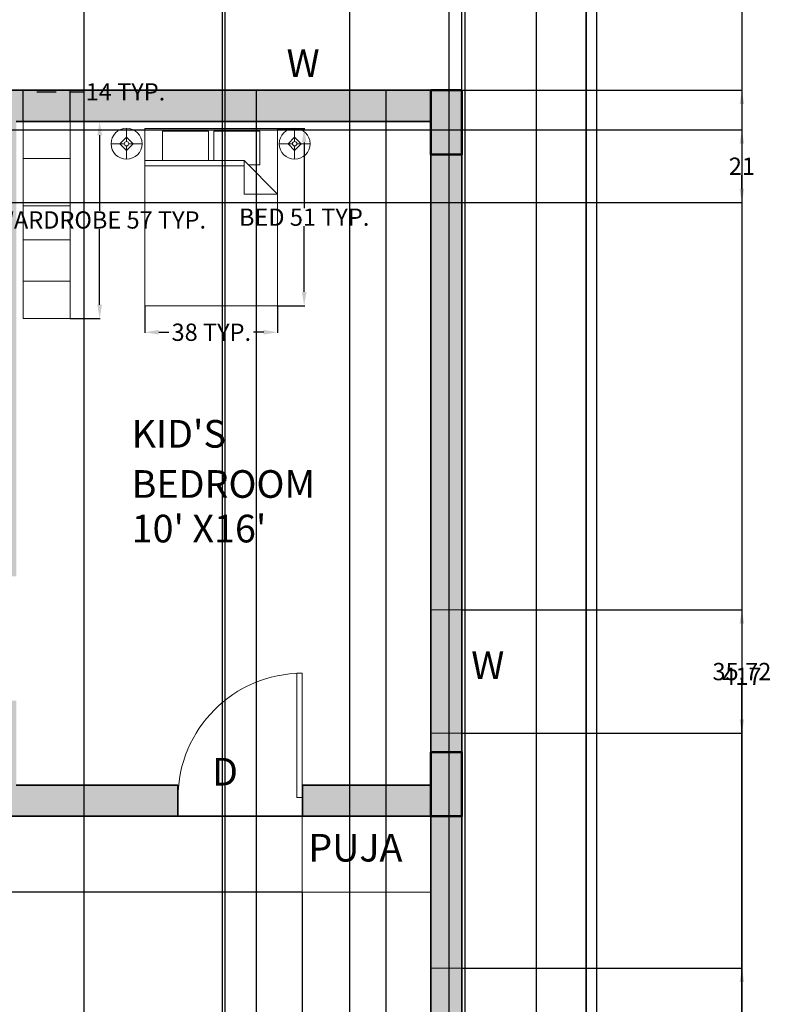
# Model space of a CAD drawing. Units: inches. Extents: x 460 to 1030, y -658 to 271.
# Tile 9 of 10: x 813 to 1030, y -174 to 111. Entities that reach past the tile are written whole.
import ezdxf

# ---------------------------------------------------------------- set-up
doc = ezdxf.new("R2010")
doc.units = ezdxf.units.IN
doc.header["$MEASUREMENT"] = 0
for name, color, linetype, lineweight in [('A-ANNO-DIMS', 2, 'Continuous', 18), ('A-ANNO-TEXT', 7, 'Continuous', 18), ('A-AREA-IDEN', 7, 'Continuous', 25), ('A-COLS', 7, 'Continuous', 50), ('A-DOOR', 3, 'Continuous', 20), ('A-FLOR-CASE', 9, 'Continuous', 18), ('A-FURN', 8, 'Continuous', 18), ('A-GLAZ', 4, 'Continuous', 20), ('A-GLAZ-PATT', 4, 'Continuous', 13), ('A-WALL', 7, 'Continuous', 35), ('A-WALL-PATT', 5, 'Continuous', 13), ('C-PROP', 7, 'Continuous', 25)]:
    doc.layers.add(name, color=color, linetype=linetype, lineweight=lineweight)
doc.layers.add('A-COLS-PATT', color=7, linetype='Continuous', lineweight=13, true_color=0xffffff)
doc.styles.get("Standard").update_dxf_attribs({"font": 'arial.ttf'})
doc.dimstyles.get("Standard").update_dxf_attribs({"dimtxt": 5, "dimasz": 4, "dimexe": 0.18, "dimexo": 0.0625, "dimgap": 0.09, "dimtad": 0, "dimtih": 1, "dimtoh": 1, "dimdec": 1, "dimzin": 0, "dimdsep": 46, "dimlunit": 4, "dimtxsty": 'Standard', "dimcen": 0.09, "dimadec": 0, "dimazin": 0, "dimtfac": 1, "dimtdec": 1, "dimtofl": 0, "dimtmove": 0, "dimatfit": 3, "dimfxl": 1, "dimtolj": 1, "dimtzin": 0, "dimarcsym": 0})

# ---------------------------------------------------------------- blocks, each defined once
blk = doc.blocks.new('Bed - Queen')
for p, q in [((0, -80.00003), (0, 0)), ((0, 0), (59.99999, 0)), ((59.99999, 0), (59.99999, -80.00003)), ((7.99999, -1.2), (28.79998, -1.2)), ((7.99999, -14.4), (7.99999, -1.2)), ((28.79998, -1.2), (28.79998, -14.4)), ((31.19999, -1.2), (51.99999, -1.2)), ((31.19999, -14.4), (31.19999, -1.2)), ((51.99999, -1.2), (51.99999, -16.4)), ((0, -14.4), (44.8, -14.4)), ((44.8, -16.8), (0, -16.8)), ((59.99999, -29.6), (44.8, -14.4)), ((44.8, -14.4), (44.8, -29.6)), ((51.99999, -16.4), (46.79936, -16.4)), ((44.8, -29.6), (59.99999, -29.6)), ((59.99999, -80.00003), (0, -80.00003))]:
    blk.add_line(p, q)
blk = doc.blocks.new('Lamp - Table')
for p, q in [((0, 7), (0, 1)), ((-1, 0), (-7, 0)), ((0, 3), (-3, 0)), ((-3, 0), (0, -3)), ((3, 0), (0, 3)), ((0, -3), (3, 0)), ((1, 0), (7, 0)), ((0, -1), (0, -7))]:
    blk.add_line(p, q)
for radius in [7, 1]:
    blk.add_circle((0, 0), radius)
blk = doc.blocks.new('*U2')
for p, q in [((0, 0), (0, -6)), ((40, 0), (40, -6))]:
    blk.add_line(p, q)
blk.add_lwpolyline([(0, 0), (0, 40), (1.75, 40), (1.75, 0)], close=True)
blk.add_arc((0, 0), 40, 0, 90)
blk = doc.blocks.new('BEDROOM-STORAGE-UNIT')
for p, q in [((10.68, 0), (10.68, -13.59)), ((24.45, 0), (24.45, -13.59)), ((34.21, 0), (34.21, -13.59)), ((46.22, 0), (46.22, -13.59))]:
    blk.add_line(p, q)
blk.add_lwpolyline([(0, 0), (57.01, 0), (57.01, -13.59), (0, -13.59)], close=True)
blk = doc.blocks.new('COL-RECT-TYPE-A')
blk.add_lwpolyline([(0, 0), (9, 0), (9, -18.58), (0, -18.58)], close=True)
blk = doc.blocks.new('*D25')
at = {"layer": 'A-ANNO-DIMS', "color": 0, "lineweight": -2, "transparency": 16777216}
for p, q in [((887.53, 79.18), (895.33, 79.18)), ((895.15, 75.18), (895.15, 56.22)), ((895.15, 31.97), (895.15, 50.93)), ((887.53, 27.97), (895.33, 27.97))]:
    blk.add_line(p, q, dxfattribs=at)
at = {"layer": 'A-ANNO-DIMS', "color": 0, "transparency": 16777216}
for points in [[(894.48, 75.18), (895.82, 75.18), (895.15, 79.18)], [(894.48, 31.97), (895.82, 31.97), (895.15, 27.97)]]:
    blk.add_solid(points, dxfattribs=at)
at = {"layer": 'Defpoints', "color": 0, "transparency": 16777216}
for p in [(887.47, 79.18), (895.15, 79.18), (887.47, 27.97)]:
    blk.add_point(p, dxfattribs=at)
at = {"layer": 'A-ANNO-DIMS', "color": 0, "transparency": 16777216, "insert": (895.15, 53.58), "char_height": 5, "attachment_point": 5}
blk.add_mtext('\\A1;BED 51 TYP.', dxfattribs=at)
blk = doc.blocks.new('*D26')
at = {"layer": 'A-ANNO-DIMS', "color": 0, "lineweight": -2, "transparency": 16777216}
for p, q in [((849.06, 27.91), (849.06, 20.11)), ((887.47, 27.91), (887.47, 20.11)), ((853.06, 20.29), (856.01, 20.29)), ((883.47, 20.29), (880.52, 20.29))]:
    blk.add_line(p, q, dxfattribs=at)
at = {"layer": 'A-ANNO-DIMS', "color": 0, "transparency": 16777216}
for points in [[(853.06, 20.96), (853.06, 19.62), (849.06, 20.29)], [(883.47, 20.96), (883.47, 19.62), (887.47, 20.29)]]:
    blk.add_solid(points, dxfattribs=at)
at = {"layer": 'Defpoints', "color": 0, "transparency": 16777216}
for p in [(849.06, 27.97), (887.47, 27.97), (887.47, 20.29)]:
    blk.add_point(p, dxfattribs=at)
at = {"layer": 'A-ANNO-DIMS', "color": 0, "transparency": 16777216, "insert": (868.27, 20.29), "char_height": 5, "attachment_point": 5}
blk.add_mtext('\\A1;38 TYP.', dxfattribs=at)
blk = doc.blocks.new('*D27')
at = {"layer": 'A-ANNO-DIMS', "color": 0, "lineweight": -2, "transparency": 16777216}
for p, q in [((827.46, 81.27), (836.13, 81.27)), ((835.95, 77.27), (835.95, 55.44)), ((835.95, 28.26), (835.95, 50.09)), ((827.46, 24.26), (836.13, 24.26))]:
    blk.add_line(p, q, dxfattribs=at)
at = {"layer": 'A-ANNO-DIMS', "color": 0, "transparency": 16777216}
for points in [[(835.28, 77.27), (836.62, 77.27), (835.95, 81.27)], [(835.28, 28.26), (836.62, 28.26), (835.95, 24.26)]]:
    blk.add_solid(points, dxfattribs=at)
at = {"layer": 'Defpoints', "color": 0, "transparency": 16777216}
for p in [(827.4, 81.27), (827.4, 24.26), (835.95, 24.26)]:
    blk.add_point(p, dxfattribs=at)
at = {"layer": 'A-ANNO-DIMS', "color": 0, "transparency": 16777216, "insert": (835.95, 52.77), "char_height": 5, "attachment_point": 5}
blk.add_mtext('\\A1;WARDROBE 57 TYP.', dxfattribs=at)
blk = doc.blocks.new('*D28')
at = {"layer": 'A-ANNO-DIMS', "color": 0, "lineweight": -2, "transparency": 16777216}
for p, q in [((813.8, 81.34), (813.8, 90.01)), ((817.8, 89.83), (823.4, 89.83)), ((827.4, 81.34), (827.4, 90.01)), ((827.4, 89.83), (831.4, 89.83))]:
    blk.add_line(p, q, dxfattribs=at)
at = {"layer": 'A-ANNO-DIMS', "color": 0, "transparency": 16777216}
for points in [[(817.8, 90.49), (817.8, 89.16), (813.8, 89.83)], [(823.4, 90.49), (823.4, 89.16), (827.4, 89.83)]]:
    blk.add_solid(points, dxfattribs=at)
at = {"layer": 'Defpoints', "color": 0, "transparency": 16777216}
for p in [(827.4, 89.83), (813.8, 81.27), (827.4, 81.27)]:
    blk.add_point(p, dxfattribs=at)
at = {"layer": 'A-ANNO-DIMS', "color": 0, "transparency": 16777216, "insert": (843.42, 89.83), "char_height": 5, "attachment_point": 5}
blk.add_mtext('\\A1;14 TYP.', dxfattribs=at)
blk = doc.blocks.new('*D41')
at = {"layer": 'A-ANNO-DIMS', "color": 0, "lineweight": -2, "transparency": 16777216}
for p, q in [((979.86, 129.27), (1022.03, 129.27)), ((1021.85, 125.27), (1021.85, -76.63)), ((1021.85, -283.73), (1021.85, -81.83)), ((940.86, -287.73), (1022.03, -287.73))]:
    blk.add_line(p, q, dxfattribs=at)
at = {"layer": 'A-ANNO-DIMS', "color": 0, "transparency": 16777216}
for points in [[(1021.18, 125.27), (1022.51, 125.27), (1021.85, 129.27)], [(1021.18, -283.73), (1022.51, -283.73), (1021.85, -287.73)]]:
    blk.add_solid(points, dxfattribs=at)
at = {"layer": 'Defpoints', "color": 0, "transparency": 16777216}
for p in [(979.8, 129.27), (1021.85, 129.27), (940.8, -287.73)]:
    blk.add_point(p, dxfattribs=at)
at = {"layer": 'A-ANNO-DIMS', "color": 0, "transparency": 16777216, "insert": (1021.85, -79.23), "char_height": 5, "attachment_point": 5}
blk.add_mtext('\\A1;417', dxfattribs=at)
blk = doc.blocks.new('*D43')
at = {"layer": 'A-ANNO-DIMS', "color": 0, "lineweight": -2, "transparency": 16777216}
for p, q in [((562.8, 90.34), (562.8, 267.89)), ((940.8, 90.34), (940.8, 267.89)), ((566.8, 267.71), (746.18, 267.71)), ((936.8, 267.71), (757.41, 267.71))]:
    blk.add_line(p, q, dxfattribs=at)
at = {"layer": 'A-ANNO-DIMS', "color": 0, "transparency": 16777216}
for points in [[(566.8, 268.38), (566.8, 267.04), (562.8, 267.71)], [(936.8, 268.38), (936.8, 267.04), (940.8, 267.71)]]:
    blk.add_solid(points, dxfattribs=at)
at = {"layer": 'Defpoints', "color": 0, "transparency": 16777216}
for p in [(940.8, 267.71), (562.8, 90.27), (940.8, 90.27)]:
    blk.add_point(p, dxfattribs=at)
at = {"layer": 'A-ANNO-DIMS', "color": 0, "transparency": 16777216, "insert": (751.8, 267.71), "char_height": 5, "attachment_point": 5}
blk.add_mtext('\\A1;378', dxfattribs=at)
blk = doc.blocks.new('*D44')
at = {"layer": 'A-ANNO-DIMS', "color": 0, "lineweight": -2, "transparency": 16777216}
for p, q in [((940.86, 90.27), (1022.03, 90.27)), ((1021.85, 86.27), (1021.85, -195.08)), ((1021.85, -481.73), (1021.85, -200.37)), ((979.86, -485.73), (1022.03, -485.73))]:
    blk.add_line(p, q, dxfattribs=at)
at = {"layer": 'A-ANNO-DIMS', "color": 0, "transparency": 16777216}
for points in [[(1021.18, 86.27), (1022.51, 86.27), (1021.85, 90.27)], [(1021.18, -481.73), (1022.51, -481.73), (1021.85, -485.73)]]:
    blk.add_solid(points, dxfattribs=at)
at = {"layer": 'Defpoints', "color": 0, "transparency": 16777216}
for p in [(940.8, 90.27), (979.8, -485.73), (1021.85, -485.73)]:
    blk.add_point(p, dxfattribs=at)
at = {"layer": 'A-ANNO-DIMS', "color": 0, "transparency": 16777216, "insert": (1021.85, -197.73), "char_height": 5, "attachment_point": 5}
blk.add_mtext('\\A1;576', dxfattribs=at)
blk = doc.blocks.new('*D45')
at = {"layer": 'A-ANNO-DIMS', "color": 0, "lineweight": -2, "transparency": 16777216}
for p, q in [((976.8, 126.21), (976.8, -654.61)), ((940.8, 90.21), (940.8, -654.61)), ((944.8, -654.43), (955.13, -654.43)), ((972.8, -654.43), (962.46, -654.43))]:
    blk.add_line(p, q, dxfattribs=at)
at = {"layer": 'A-ANNO-DIMS', "color": 0, "transparency": 16777216}
for points in [[(944.8, -653.77), (944.8, -655.1), (940.8, -654.43)], [(972.8, -653.77), (972.8, -655.1), (976.8, -654.43)]]:
    blk.add_solid(points, dxfattribs=at)
at = {"layer": 'Defpoints', "color": 0, "transparency": 16777216}
for p in [(976.8, 126.27), (940.8, 90.27), (976.8, -654.43)]:
    blk.add_point(p, dxfattribs=at)
at = {"layer": 'A-ANNO-DIMS', "color": 0, "transparency": 16777216, "insert": (958.8, -654.43), "char_height": 5, "attachment_point": 5}
blk.add_mtext('\\A1;36', dxfattribs=at)
blk = doc.blocks.new('*D46')
at = {"layer": 'A-ANNO-DIMS', "color": 0, "lineweight": -2, "transparency": 16777216}
for p, q in [((936.98, 127.21), (936.98, -654.61)), ((962.32, 127.21), (962.32, -654.61)), ((932.98, -654.43), (928.98, -654.43)), ((966.32, -654.43), (970.32, -654.43))]:
    blk.add_line(p, q, dxfattribs=at)
at = {"layer": 'A-ANNO-DIMS', "color": 0, "transparency": 16777216}
for points in [[(932.98, -653.77), (932.98, -655.1), (936.98, -654.43)], [(966.32, -653.77), (966.32, -655.1), (962.32, -654.43)]]:
    blk.add_solid(points, dxfattribs=at)
at = {"layer": 'Defpoints', "color": 0, "transparency": 16777216}
for p in [(936.98, 127.27), (962.32, 127.27), (962.32, -654.43)]:
    blk.add_point(p, dxfattribs=at)
at = {"layer": 'A-ANNO-DIMS', "color": 0, "transparency": 16777216, "insert": (949.65, -654.43), "char_height": 5, "attachment_point": 5}
blk.add_mtext('\\A1;25.346', dxfattribs=at)
blk = doc.blocks.new('*D47')
at = {"layer": 'A-ANNO-DIMS', "color": 0, "lineweight": -2, "transparency": 16777216}
for p, q in [((962.32, 129.21), (962.32, -654.61)), ((979.8, 129.21), (979.8, -654.61)), ((966.32, -654.43), (975.8, -654.43)), ((979.8, -654.43), (983.8, -654.43))]:
    blk.add_line(p, q, dxfattribs=at)
at = {"layer": 'A-ANNO-DIMS', "color": 0, "transparency": 16777216}
for points in [[(966.32, -653.77), (966.32, -655.1), (962.32, -654.43)], [(975.8, -653.77), (975.8, -655.1), (979.8, -654.43)]]:
    blk.add_solid(points, dxfattribs=at)
at = {"layer": 'Defpoints', "color": 0, "transparency": 16777216}
for p in [(962.32, 129.27), (979.8, 129.27), (979.8, -654.43)]:
    blk.add_point(p, dxfattribs=at)
at = {"layer": 'A-ANNO-DIMS', "color": 0, "transparency": 16777216, "insert": (994.02, -654.43), "char_height": 5, "attachment_point": 5}
blk.add_mtext('\\A1;17.474', dxfattribs=at)
blk = doc.blocks.new('*D48')
at = {"layer": 'A-ANNO-DIMS', "color": 0, "lineweight": -2, "transparency": 16777216}
for p, q in [((799.88, -611.66), (799.88, 267.89)), ((941.7, -611.66), (941.7, 267.89)), ((803.88, 267.71), (860.58, 267.71)), ((937.7, 267.71), (881, 267.71))]:
    blk.add_line(p, q, dxfattribs=at)
at = {"layer": 'A-ANNO-DIMS', "color": 0, "transparency": 16777216}
for points in [[(803.88, 268.38), (803.88, 267.04), (799.88, 267.71)], [(937.7, 268.38), (937.7, 267.04), (941.7, 267.71)]]:
    blk.add_solid(points, dxfattribs=at)
at = {"layer": 'Defpoints', "color": 0, "transparency": 16777216}
for p in [(941.7, 267.71), (799.88, -611.73), (941.7, -611.73)]:
    blk.add_point(p, dxfattribs=at)
at = {"layer": 'A-ANNO-DIMS', "color": 0, "transparency": 16777216, "insert": (870.79, 267.71), "char_height": 5, "attachment_point": 5}
blk.add_mtext('\\A1;141.82', dxfattribs=at)
blk = doc.blocks.new('*D49')
at = {"layer": 'A-ANNO-DIMS', "color": 0, "lineweight": -2, "transparency": 16777216}
for p, q in [((941.7, -608.66), (941.7, 267.89)), ((976.8, -608.66), (976.8, 267.89)), ((945.7, 267.71), (953.15, 267.71)), ((972.8, 267.71), (965.35, 267.71))]:
    blk.add_line(p, q, dxfattribs=at)
at = {"layer": 'A-ANNO-DIMS', "color": 0, "transparency": 16777216}
for points in [[(945.7, 268.38), (945.7, 267.04), (941.7, 267.71)], [(972.8, 268.38), (972.8, 267.04), (976.8, 267.71)]]:
    blk.add_solid(points, dxfattribs=at)
at = {"layer": 'Defpoints', "color": 0, "transparency": 16777216}
for p in [(976.8, 267.71), (941.7, -608.73), (976.8, -608.73)]:
    blk.add_point(p, dxfattribs=at)
at = {"layer": 'A-ANNO-DIMS', "color": 0, "transparency": 16777216, "insert": (959.25, 267.71), "char_height": 5, "attachment_point": 5}
blk.add_mtext('\\A1;35.1', dxfattribs=at)
blk = doc.blocks.new('*D52')
at = {"layer": 'A-ANNO-DIMS', "color": 0, "lineweight": -2, "transparency": 16777216}
for p, q in [((872.3, -281.66), (872.3, 267.89)), ((908.35, -281.66), (908.35, 267.89)), ((876.3, 267.71), (879.84, 267.71)), ((904.35, 267.71), (900.81, 267.71))]:
    blk.add_line(p, q, dxfattribs=at)
at = {"layer": 'A-ANNO-DIMS', "color": 0, "transparency": 16777216}
for points in [[(876.3, 268.38), (876.3, 267.04), (872.3, 267.71)], [(904.35, 268.38), (904.35, 267.04), (908.35, 267.71)]]:
    blk.add_solid(points, dxfattribs=at)
at = {"layer": 'Defpoints', "color": 0, "transparency": 16777216}
for p in [(908.35, 267.71), (872.3, -281.73), (908.35, -281.73)]:
    blk.add_point(p, dxfattribs=at)
at = {"layer": 'A-ANNO-DIMS', "color": 0, "transparency": 16777216, "insert": (890.32, 267.71), "char_height": 5, "attachment_point": 5}
blk.add_mtext('\\A1;36.045', dxfattribs=at)
blk = doc.blocks.new('*D54')
at = {"layer": 'A-ANNO-DIMS', "color": 0, "lineweight": -2, "transparency": 16777216}
for p, q in [((894.61, -141.78), (894.61, -654.61)), ((931.8, -141.78), (931.8, -654.61)), ((898.61, -654.43), (904.68, -654.43)), ((927.8, -654.43), (921.73, -654.43))]:
    blk.add_line(p, q, dxfattribs=at)
at = {"layer": 'A-ANNO-DIMS', "color": 0, "transparency": 16777216}
for points in [[(898.61, -653.77), (898.61, -655.1), (894.61, -654.43)], [(927.8, -653.77), (927.8, -655.1), (931.8, -654.43)]]:
    blk.add_solid(points, dxfattribs=at)
at = {"layer": 'Defpoints', "color": 0, "transparency": 16777216}
for p in [(894.61, -141.72), (931.8, -141.72), (931.8, -654.43)]:
    blk.add_point(p, dxfattribs=at)
at = {"layer": 'A-ANNO-DIMS', "color": 0, "transparency": 16777216, "insert": (913.2, -654.43), "char_height": 5, "attachment_point": 5}
blk.add_mtext('\\A1;37.18', dxfattribs=at)
blk = doc.blocks.new('*D55')
at = {"layer": 'A-ANNO-DIMS', "color": 0, "lineweight": -2, "transparency": 16777216}
for p, q in [((894.56, -119.73), (470.68, -119.73)), ((470.86, -123.73), (470.86, -128.08)), ((470.86, -137.72), (470.86, -133.37)), ((894.55, -141.72), (470.68, -141.72))]:
    blk.add_line(p, q, dxfattribs=at)
at = {"layer": 'A-ANNO-DIMS', "color": 0, "transparency": 16777216}
for points in [[(470.19, -123.73), (471.52, -123.73), (470.86, -119.73)], [(470.19, -137.72), (471.52, -137.72), (470.86, -141.72)]]:
    blk.add_solid(points, dxfattribs=at)
at = {"layer": 'Defpoints', "color": 0, "transparency": 16777216}
for p in [(470.86, -119.73), (894.62, -119.73), (894.61, -141.72)]:
    blk.add_point(p, dxfattribs=at)
at = {"layer": 'A-ANNO-DIMS', "color": 0, "transparency": 16777216, "insert": (470.86, -130.72), "char_height": 5, "attachment_point": 5}
blk.add_mtext('\\A1;21.995', dxfattribs=at)
blk = doc.blocks.new('*D59')
at = {"layer": 'A-ANNO-DIMS', "color": 0, "lineweight": -2, "transparency": 16777216}
for p, q in [((940.86, -60), (1022.03, -60)), ((1021.85, -64), (1021.85, -75.22)), ((1021.85, -91.73), (1021.85, -80.51)), ((940.86, -95.73), (1022.03, -95.73))]:
    blk.add_line(p, q, dxfattribs=at)
at = {"layer": 'A-ANNO-DIMS', "color": 0, "transparency": 16777216}
for points in [[(1021.18, -64), (1022.51, -64), (1021.85, -60)], [(1021.18, -91.73), (1022.51, -91.73), (1021.85, -95.73)]]:
    blk.add_solid(points, dxfattribs=at)
at = {"layer": 'Defpoints', "color": 0, "transparency": 16777216}
for p in [(940.8, -60), (940.8, -95.73), (1021.85, -95.73)]:
    blk.add_point(p, dxfattribs=at)
at = {"layer": 'A-ANNO-DIMS', "color": 0, "transparency": 16777216, "insert": (1021.85, -77.87), "char_height": 5, "attachment_point": 5}
blk.add_mtext('\\A1;35.72', dxfattribs=at)
blk = doc.blocks.new('*D60')
at = {"layer": 'A-ANNO-DIMS', "color": 0, "lineweight": -2, "transparency": 16777216}
for p, q in [((940.86, -163.66), (1022.03, -163.66)), ((1021.85, -167.66), (1021.85, -194.33)), ((1021.85, -226.29), (1021.85, -199.62)), ((940.86, -230.29), (1022.03, -230.29))]:
    blk.add_line(p, q, dxfattribs=at)
at = {"layer": 'A-ANNO-DIMS', "color": 0, "transparency": 16777216}
for points in [[(1021.18, -167.66), (1022.51, -167.66), (1021.85, -163.66)], [(1021.18, -226.29), (1022.51, -226.29), (1021.85, -230.29)]]:
    blk.add_solid(points, dxfattribs=at)
at = {"layer": 'Defpoints', "color": 0, "transparency": 16777216}
for p in [(940.8, -163.66), (940.8, -230.29), (1021.85, -230.29)]:
    blk.add_point(p, dxfattribs=at)
at = {"layer": 'A-ANNO-DIMS', "color": 0, "transparency": 16777216, "insert": (1021.85, -196.98), "char_height": 5, "attachment_point": 5}
blk.add_mtext('\\A1;66.64', dxfattribs=at)
blk = doc.blocks.new('*D69')
at = {"layer": 'A-ANNO-DIMS', "color": 0, "lineweight": -2, "transparency": 16777216}
for p, q in [((881.27, 90.21), (881.27, -654.61)), ((918.77, 90.21), (918.77, -654.61)), ((885.27, -654.43), (893.42, -654.43)), ((914.77, -654.43), (906.62, -654.43))]:
    blk.add_line(p, q, dxfattribs=at)
at = {"layer": 'A-ANNO-DIMS', "color": 0, "transparency": 16777216}
for points in [[(885.27, -653.77), (885.27, -655.1), (881.27, -654.43)], [(914.77, -653.77), (914.77, -655.1), (918.77, -654.43)]]:
    blk.add_solid(points, dxfattribs=at)
at = {"layer": 'Defpoints', "color": 0, "transparency": 16777216}
for p in [(881.27, 90.27), (918.77, 90.27), (918.77, -654.43)]:
    blk.add_point(p, dxfattribs=at)
at = {"layer": 'A-ANNO-DIMS', "color": 0, "transparency": 16777216, "insert": (900.02, -654.43), "char_height": 5, "attachment_point": 5}
blk.add_mtext('\\A1;37.5', dxfattribs=at)
blk = doc.blocks.new('*D71')
at = {"layer": 'A-ANNO-DIMS', "color": 0, "lineweight": -2, "transparency": 16777216}
for p, q in [((831.43, -281.66), (831.43, 267.89)), ((871.46, -281.66), (871.46, 267.89)), ((835.43, 267.71), (840.88, 267.71)), ((867.46, 267.71), (862.01, 267.71))]:
    blk.add_line(p, q, dxfattribs=at)
at = {"layer": 'A-ANNO-DIMS', "color": 0, "transparency": 16777216}
for points in [[(835.43, 268.38), (835.43, 267.04), (831.43, 267.71)], [(867.46, 268.38), (867.46, 267.04), (871.46, 267.71)]]:
    blk.add_solid(points, dxfattribs=at)
at = {"layer": 'Defpoints', "color": 0, "transparency": 16777216}
for p in [(871.46, 267.71), (831.43, -281.73), (871.46, -281.73)]:
    blk.add_point(p, dxfattribs=at)
at = {"layer": 'A-ANNO-DIMS', "color": 0, "transparency": 16777216, "insert": (851.44, 267.71), "char_height": 5, "attachment_point": 5}
blk.add_mtext('\\A1;40.026', dxfattribs=at)
blk = doc.blocks.new('*D73')
at = {"layer": 'A-ANNO-DIMS', "color": 0, "lineweight": -2, "transparency": 16777216}
for p, q in [((748.86, 78.81), (1022.03, 78.81)), ((1021.85, 74.81), (1021.85, 70.92)), ((1021.85, 61.81), (1021.85, 65.71)), ((748.86, 57.81), (1022.03, 57.81))]:
    blk.add_line(p, q, dxfattribs=at)
at = {"layer": 'A-ANNO-DIMS', "color": 0, "transparency": 16777216}
for points in [[(1021.18, 74.81), (1022.51, 74.81), (1021.85, 78.81)], [(1021.18, 61.81), (1022.51, 61.81), (1021.85, 57.81)]]:
    blk.add_solid(points, dxfattribs=at)
at = {"layer": 'Defpoints', "color": 0, "transparency": 16777216}
for p in [(748.8, 78.81), (748.8, 57.81), (1021.85, 57.81)]:
    blk.add_point(p, dxfattribs=at)
at = {"layer": 'A-ANNO-DIMS', "color": 0, "transparency": 16777216, "insert": (1021.85, 68.31), "char_height": 5, "attachment_point": 5}
blk.add_mtext('\\A1;21', dxfattribs=at)

msp = doc.modelspace()

# ---------------------------------------------------------------- hatches: boundary and pattern name
at = {"layer": 'A-COLS-PATT'}
h = msp.add_hatch(color=256, dxfattribs=at)
h.dxf.hatch_style = 1
h.paths.add_polyline_path([(571.7961, 90.2738), (562.7961, 90.2738), (562.7961, 71.6966), (571.7961, 71.6966)])
h.paths.add_polyline_path([(700.7961, 90.2738), (691.7961, 90.2738), (691.7961, 71.6966), (700.7961, 71.6966)])
h.paths.add_polyline_path([(811.7961, 90.2738), (802.7961, 90.2738), (802.7961, 71.6966), (811.7961, 71.6966)])
h.paths.add_polyline_path([(940.7961, 90.2738), (931.7961, 90.2738), (931.7961, 71.6966), (940.7961, 71.6966)])
h.paths.add_polyline_path([(940.7961, -101.149), (931.7961, -101.149), (931.7961, -119.7262), (940.7961, -119.7262)])
h.paths.add_polyline_path([(940.7961, -268.3723), (931.7961, -268.3723), (931.7961, -287.7262), (940.7961, -287.7262)])
h.paths.add_polyline_path([(803.0275, -281.7262), (789.8237, -281.7262), (789.8237, -287.7262), (803.0275, -287.7262)])
h.paths.add_polyline_path([(700.7961, -303.809), (691.7961, -303.809), (691.7961, -323.8443), (700.7961, -323.8443)])
h.paths.add_polyline_path([(571.7961, -303.809), (562.7961, -303.809), (562.7961, -323.8443), (571.7961, -323.8443)])
h.paths.add_polyline_path([(571.7961, -413.1453), (562.7961, -413.1453), (562.7961, -432.4659), (571.7961, -432.4659)])
h.paths.add_polyline_path([(571.7961, -101.149), (562.7961, -101.149), (562.7961, -119.7262), (571.7961, -119.7262)])
h.paths.add_polyline_path([(700.7961, -101.0985), (691.7961, -101.0985), (691.7961, -119.7262), (700.7961, -119.7262)])
h.paths.add_polyline_path([(811.7961, -101.149), (802.7961, -101.149), (802.7961, -119.7262), (811.7961, -119.7262)])
at = {"layer": 'A-GLAZ-PATT'}
h = msp.add_hatch(color=256, dxfattribs=at)
h.dxf.hatch_style = 1
h.paths.add_polyline_path([(571.7961, -343.9041), (562.7961, -343.9041), (562.7961, -384.3969), (571.7961, -384.3969)])
h.paths.add_polyline_path([(571.7961, -143.2895), (562.7961, -143.2895), (562.7961, -168.3798), (571.7961, -168.3798)])
h.paths.add_polyline_path([(571.7961, -49.2966), (562.7961, -49.2966), (562.7961, -90.3192), (571.7961, -90.3192)])
h.paths.add_polyline_path([(666.4584, 90.2738), (634.2742, 90.2738), (634.2742, 81.2738), (666.4584, 81.2738)])
h.paths.add_polyline_path([(742.1779, 90.2738), (713.201, 90.2738), (713.201, 81.2738), (742.1779, 81.2738)])
h.paths.add_polyline_path([(797.2395, 90.2738), (768.2626, 90.2738), (768.2626, 81.2738), (797.2395, 81.2738)])
h.paths.add_polyline_path([(918.7723, 90.2738), (881.2728, 90.2738), (881.2728, 81.2738), (918.7723, 81.2738)])
h.paths.add_polyline_path([(940.7961, -60.0042), (931.7961, -60.0042), (931.7961, -95.7262), (940.7961, -95.7262)])
h.paths.add_polyline_path([(940.7961, -163.6558), (931.7961, -163.6558), (931.7961, -230.2946), (940.7961, -230.2946)])
h.paths.add_polyline_path([(913.7961, -331.7262), (835.7961, -331.7262), (835.7961, -332.7262), (913.7961, -332.7262)])
h.paths.add_polyline_path([(871.4559, -281.7262), (831.4302, -281.7262), (831.4302, -287.7262), (871.4559, -287.7262)])
h.paths.add_polyline_path([(774.8576, -281.7262), (716.7073, -281.7262), (716.7073, -287.7262), (774.8576, -287.7262)])
at = {"layer": 'A-WALL-PATT'}
h = msp.add_hatch(color=256, dxfattribs=at)
h.dxf.hatch_style = 1
h.paths.add_polyline_path([(634.2742, 90.2738), (571.7961, 90.2738), (571.7961, 81.2738), (634.2742, 81.2738)])
h.paths.add_polyline_path([(691.7961, 90.2738), (666.4584, 90.2738), (666.4584, 81.2738), (691.7961, 81.2738)])
h.paths.add_polyline_path([(713.201, 90.2738), (700.7961, 90.2738), (700.7961, 81.2738), (713.201, 81.2738)])
h.paths.add_polyline_path([(748.7961, 90.2738), (742.1779, 90.2738), (742.1779, 81.2738), (748.7961, 81.2738)])
h.paths.add_polyline_path([(768.2626, 90.2738), (754.7961, 90.2738), (754.7961, 81.2738), (768.2626, 81.2738)])
h.paths.add_polyline_path([(802.7961, 90.2738), (797.2395, 90.2738), (797.2395, 81.2738), (802.7961, 81.2738)])
h.paths.add_polyline_path([(881.2728, 90.2738), (811.7961, 90.2738), (811.7961, 81.2738), (881.2728, 81.2738)])
h.paths.add_polyline_path([(931.7961, 90.2738), (918.7723, 90.2738), (918.7723, 81.2738), (931.7961, 81.2738)])
h.paths.add_polyline_path([(940.7961, 71.6966), (931.7961, 71.6966), (931.7961, -60.0042), (940.7961, -60.0042)])
h.paths.add_polyline_path([(940.7961, -95.7262), (931.7961, -95.7262), (931.7961, -101.149), (940.7961, -101.149)])
h.paths.add_polyline_path([(931.7961, -110.7262), (894.6225, -110.7262), (894.6225, -119.7262), (931.7961, -119.7262)])
h.paths.add_polyline_path([(858.6225, -110.7262), (811.7961, -110.7262), (811.7961, -119.7262), (858.6225, -119.7262)])
h.paths.add_polyline_path([(940.7961, -119.7262), (931.7961, -119.7262), (931.7961, -141.7212), (931.7961, -163.6558), (940.7961, -163.6558)])
h.paths.add_polyline_path([(940.7961, -230.2946), (931.7961, -230.2946), (931.7961, -268.3723), (940.7961, -268.3723)])
h.paths.add_polyline_path([(931.7961, -281.7262), (908.3452, -281.7262), (908.3452, -285.0181), (908.3452, -287.7262), (931.7961, -287.7262)])
h.paths.add_polyline_path([(831.4302, -281.7262), (803.0275, -281.7262), (803.0275, -287.7262), (808.7961, -287.7262), (808.7961, -339.7262), (811.7961, -339.7262), (811.7961, -287.7262), (831.4302, -287.7262)])
h.paths.add_polyline_path([(789.8237, -281.7262), (774.8576, -281.7262), (774.8576, -287.7262), (789.8237, -287.7262)])
h.paths.add_polyline_path([(716.7073, -281.7262), (700.7961, -281.7262), (700.7961, -271.1977), (691.7961, -271.1977), (691.7961, -281.7262), (682.4735, -281.7262), (682.4735, -287.7262), (691.7961, -287.7262), (691.7961, -303.809), (700.7961, -303.809), (700.7961, -287.7262), (716.7073, -287.7262)])
h.paths.add_polyline_path([(700.7961, -323.8443), (691.7961, -323.8443), (691.7961, -413.1453), (700.7961, -413.1453)])
h.paths.add_polyline_path([(940.7961, -287.7262), (937.7961, -287.7262), (937.7961, -339.7262), (940.7961, -339.7262)])
h.paths.add_polyline_path([(937.7961, -336.7262), (811.7961, -336.7262), (811.7961, -339.7262), (937.7961, -339.7262)])
h.paths.add_polyline_path([(835.7961, -329.7262), (811.7961, -329.7262), (811.7961, -332.7262), (835.7961, -332.7262)])
h.paths.add_polyline_path([(937.7961, -329.7262), (913.7961, -329.7262), (913.7961, -332.7262), (937.7961, -332.7262)])
h.paths.add_polyline_path([(691.7961, -419.7262), (681.4044, -419.7262), (681.4044, -428.7262), (691.7961, -428.7262)])
h.paths.add_polyline_path([(691.7961, -476.7262), (571.7961, -476.7262), (571.7961, -485.7262), (691.7961, -485.7262)])
h.paths.add_polyline_path([(571.7961, -465.0348), (568.223, -465.0348), (562.7961, -465.0348), (562.7961, -476.7262), (571.7961, -476.7262)])
h.paths.add_polyline_path([(571.7961, -432.4659), (562.7961, -432.4659), (562.7961, -441.1912), (571.7961, -441.1912)])
h.paths.add_polyline_path([(571.7961, -384.3969), (562.7961, -384.3969), (562.7961, -413.1453), (571.7961, -413.1453)])
h.paths.add_polyline_path([(571.7961, -323.8443), (562.7961, -323.8443), (562.7961, -343.9041), (571.7961, -343.9041)])
h.paths.add_polyline_path([(571.7961, -287.7262), (646.4735, -287.7262), (646.4735, -281.7262), (571.7961, -281.7262), (571.7961, -258.1542), (571.7961, -233.7262), (566.4164, -233.7262), (562.7961, -233.7262), (562.7961, -303.809), (571.7961, -303.809)])
h.paths.add_polyline_path([(571.7961, -179.7262), (691.7961, -179.7262), (691.7961, -197.5753), (700.7961, -197.5753), (700.7961, -173.7262), (647.7961, -173.7262), (647.7961, -165.5723), (643.7961, -165.5723), (643.7961, -173.7262), (571.7961, -173.7262), (571.7961, -168.3798), (562.7961, -168.3798), (562.7961, -197.7262), (571.7961, -197.7262)])
h.paths.add_polyline_path([(647.7961, -110.7262), (571.7961, -110.7262), (571.7961, -119.7262), (643.7961, -119.7262), (643.7961, -141.5723), (647.7961, -141.5723)])
h.paths.add_polyline_path([(691.7961, -110.7262), (683.7961, -110.7262), (683.7961, -114.3453), (683.7961, -119.7262), (691.7961, -119.7262)])
h.paths.add_polyline_path([(571.7961, -119.7262), (562.7961, -119.7262), (562.7961, -143.2895), (571.7961, -143.2895)])
h.paths.add_polyline_path([(571.7961, -90.3192), (562.7961, -90.3192), (562.7961, -101.149), (571.7961, -101.149)])
h.paths.add_polyline_path([(571.7961, 71.6966), (562.7961, 71.6966), (562.7961, -49.2966), (571.7961, -49.2966)])
h.paths.add_polyline_path([(700.7961, 71.6966), (691.7961, 71.6966), (691.7961, -50.298), (700.7961, -50.298)])
h.paths.add_polyline_path([(754.7961, 81.2738), (748.7961, 81.2738), (748.7961, -38.7262), (741.5908, -38.7262), (741.5908, -39.109), (741.5908, -42.7262), (748.7961, -42.7262), (748.7961, -110.7262), (754.7961, -110.7262), (754.7961, -42.7262), (773.6274, -42.7262), (773.6274, -38.7262), (754.7961, -38.7262)])
h.paths.add_polyline_path([(717.4759, -38.7262), (700.7961, -38.7262), (700.7961, -42.7262), (717.4759, -42.7262)])
h.paths.add_polyline_path([(811.7961, 71.6966), (802.7961, 71.6966), (802.7961, -50.298), (811.7961, -50.298)])
h.paths.add_polyline_path([(811.7961, -86.298), (806.4164, -86.298), (802.7961, -86.298), (802.7961, -101.149), (811.7961, -101.149)])

# ---------------------------------------------------------------- linework, layer by layer
at = {"layer": 'A-FLOR-CASE'}
msp.add_lwpolyline([(931.7961, -119.7262), (894.6132, -119.7262), (894.6132, -141.7212), (931.7961, -141.7212)], close=True, dxfattribs=at)
at = {"layer": 'A-GLAZ'}
for points in [[(918.7723, 81.2738), (881.2728, 81.2738), (881.2728, 90.2738), (918.7723, 90.2738)], [(940.7961, -95.7262), (931.7961, -95.7262), (931.7961, -60.0042), (940.7961, -60.0042)], [(940.7961, -230.2946), (931.7961, -230.2946), (931.7961, -163.6558), (940.7961, -163.6558)]]:
    msp.add_lwpolyline(points, close=True, dxfattribs=at)
at = {"layer": 'A-WALL'}
for p, q in [((940.7961, 90.2738), (562.7961, 90.2738)), ((940.7961, 90.2738), (940.7961, -281.7262)), ((931.7961, 81.2738), (811.7961, 81.2738)), ((931.7961, 81.2738), (931.7961, -281.7262)), ((858.6225, -110.7262), (811.7961, -110.7262)), ((858.6225, -110.7262), (858.6225, -119.7262)), ((931.7961, -110.7262), (894.6225, -110.7262)), ((894.6225, -119.7262), (894.6225, -110.7262)), ((940.7961, -119.7262), (647.7961, -119.7262))]:
    msp.add_line(p, q, dxfattribs=at)
at = {"layer": 'C-PROP'}
for p, q in [((979.7961, 129.2738), (979.7961, -524.7262)), ((976.7961, 126.2738), (976.7961, -466.833))]:
    msp.add_line(p, q, dxfattribs=at)

# ---------------------------------------------------------------- block references
at = {"layer": 'A-COLS'}
for p in [(931.7961, 90.2738), (931.7961, -101.149)]:
    msp.add_blockref('COL-RECT-TYPE-A', p, dxfattribs=at)
at = {"layer": 'A-DOOR', "xscale": -0.8989747935507686, "yscale": 0.8989747935507686, "zscale": 0.8989747935507686}
msp.add_blockref('*U2', (894.6087, -114.3324), dxfattribs=at)
at = {"layer": 'A-FLOR-CASE', "rotation": 270.0000000000001}
msp.add_blockref('BEDROOM-STORAGE-UNIT', (827.3963, 81.2738), dxfattribs=at)
at = {"layer": 'A-FURN', "xscale": 0.6401435689940156, "yscale": 0.6401435689940156, "zscale": 0.6401435689940156}
for name, p in [('Lamp - Table', (843.7303, 74.8233)), ('Bed - Queen', (849.0611, 79.1821)), ('Lamp - Table', (892.3951, 74.8233))]:
    msp.add_blockref(name, p, dxfattribs=at)

# ---------------------------------------------------------------- texts
at = {"layer": 'A-ANNO-TEXT'}
for s, p in [('W', (890.0479, 94.1615)), ('W', (943.4989, -80.0273)), ('D', (868.4757, -110.8395))]:
    msp.add_text(s, height=8, dxfattribs=at).set_placement(p)
at = {"layer": 'A-AREA-IDEN'}
for s, p in [("KID'S", (845.2052, -13.097)), ('BEDROOM', (845.2052, -27.6072)), ("10' X16'", (845.2052, -40.5051)), ('PUJA', (896.3422, -132.8254))]:
    msp.add_text(s, height=8, dxfattribs=at).set_placement(p)

# ---------------------------------------------------------------- dimensions: what is measured, and where the dimension line sits
at = {"layer": 'A-ANNO-DIMS'}
for base, p1, p2, override, picture, middle in [((940.7961, 267.7108), (562.7961, 90.2738), (940.7961, 90.2738), {"dimdec": 0, "dimlfac": 1, "dimrnd": 0, "dimzin": 0, "dimdsep": 46, "dimlunit": 2}, '*D43', (751.7961, 267.7108)), ((941.6978, 267.7108), (799.8801, -611.7262), (941.6978, -611.7262), {"dimdec": 2, "dimlfac": 1, "dimrnd": 0, "dimzin": 0, "dimdsep": 46, "dimlunit": 2}, '*D48', (870.7889, 267.7108)), ((871.4559, 267.7108), (831.4302, -281.7262), (871.4559, -281.7262), {"dimdec": 3, "dimlfac": 1, "dimrnd": 0, "dimzin": 0, "dimdsep": 46, "dimlunit": 2}, '*D71', (851.443, 267.7108)), ((908.3452, 267.7108), (872.2999, -281.7262), (908.3452, -281.7262), {"dimdec": 3, "dimlfac": 1, "dimrnd": 0, "dimzin": 0, "dimdsep": 46, "dimlunit": 2}, '*D52', (890.3226, 267.7108)), ((976.7961, 267.7108), (941.6978, -608.7262), (976.7961, -608.7262), {"dimdec": 1, "dimlfac": 1, "dimrnd": 0, "dimzin": 0, "dimdsep": 46, "dimlunit": 2}, '*D49', (959.247, 267.7108)), ((979.7961, -654.4339), (962.3217, 129.2738), (979.7961, 129.2738), {"dimdec": 3, "dimlfac": 1, "dimrnd": 0, "dimzin": 0, "dimdsep": 46, "dimlunit": 2}, '*D47', (994.0191, -654.4339)), ((962.3217, -654.4339), (936.9757, 127.2738), (962.3217, 127.2738), {"dimdec": 3, "dimlfac": 1, "dimrnd": 0, "dimzin": 0, "dimdsep": 46, "dimlunit": 2}, '*D46', (949.6487, -654.4339)), ((976.7961, -654.4339), (940.7961, 90.2738), (976.7961, 126.2738), {"dimdec": 0, "dimlfac": 1, "dimrnd": 0, "dimzin": 0, "dimdsep": 46, "dimlunit": 2}, '*D45', (958.7961, -654.4339)), ((918.7723, -654.4339), (881.2728, 90.2738), (918.7723, 90.2738), {"dimdec": 1, "dimlfac": 1, "dimrnd": 0, "dimzin": 0, "dimdsep": 46, "dimlunit": 2}, '*D69', (900.0226, -654.4339)), ((931.7961, -654.4339), (894.6132, -141.7212), (931.7961, -141.7212), {"dimdec": 2, "dimlfac": 1, "dimrnd": 0, "dimzin": 0, "dimdsep": 46, "dimlunit": 2}, '*D54', (913.2047, -654.4339))]:
    dim = msp.add_linear_dim(base=base, p1=p1, p2=p2, dimstyle='Standard', override=override, dxfattribs=at)
    dim.commit()
    dim.dimension.update_dxf_attribs({"geometry": picture, "text_midpoint": middle})
for base, p1, p2, override, picture, middle in [((1021.8461, 129.2738), (940.7961, -287.7262), (979.7961, 129.2738), {"dimdec": 0, "dimlfac": 1, "dimrnd": 0, "dimzin": 0, "dimdsep": 46, "dimlunit": 2}, '*D41', (1021.8461, -79.2262)), ((1021.8461, -485.7262), (940.7961, 90.2738), (979.7961, -485.7262), {"dimdec": 0, "dimlfac": 1, "dimrnd": 0, "dimzin": 0, "dimdsep": 46, "dimlunit": 2}, '*D44', (1021.8461, -197.7262)), ((1021.8461, 57.8148), (748.7961, 78.8148), (748.7961, 57.8148), {"dimdec": 0, "dimlfac": 1, "dimrnd": 0, "dimzin": 0, "dimdsep": 46, "dimlunit": 2}, '*D73', (1021.8461, 68.3148)), ((1021.8461, -95.7262), (940.7961, -60.0042), (940.7961, -95.7262), {"dimdec": 2, "dimlfac": 1, "dimrnd": 0, "dimzin": 0, "dimdsep": 46, "dimlunit": 2}, '*D59', (1021.8461, -77.8652)), ((470.8563, -119.7262), (894.6132, -141.7212), (894.6225, -119.7262), {"dimdec": 3, "dimlfac": 1, "dimrnd": 0, "dimzin": 0, "dimdsep": 46, "dimlunit": 2}, '*D55', (470.8563, -130.7237)), ((1021.8461, -230.2946), (940.7961, -163.6558), (940.7961, -230.2946), {"dimdec": 2, "dimlfac": 1, "dimrnd": 0, "dimzin": 0, "dimdsep": 46, "dimlunit": 2}, '*D60', (1021.8461, -196.9752))]:
    dim = msp.add_linear_dim(base=base, p1=p1, p2=p2, angle=90, dimstyle='Standard', override=override, dxfattribs=at)
    dim.commit()
    dim.dimension.update_dxf_attribs({"geometry": picture, "text_midpoint": middle})
for base, p1, p2, angle, text, picture, middle in [((827.3963, 89.826), (813.8022, 81.2738), (827.3963, 81.2738), 0, '<> TYP.', '*D28', (843.4201, 89.826)), ((835.9484, 24.2594), (827.3963, 81.2738), (827.3963, 24.2594), 270, 'WARDROBE <> TYP.', '*D27', (835.9484, 52.7666)), ((895.1514, 79.1821), (887.4697, 27.9706), (887.4697, 79.1821), 90, 'BED <> TYP.', '*D25', (895.1514, 53.5763))]:
    dim = msp.add_linear_dim(base=base, p1=p1, p2=p2, angle=angle, text=text, dimstyle='Standard', override={"dimdec": 0, "dimlfac": 1, "dimrnd": 0, "dimzin": 0, "dimdsep": 46, "dimlunit": 2}, dxfattribs=at)
    dim.commit()
    dim.dimension.update_dxf_attribs({"geometry": picture, "text_midpoint": middle})
dim = msp.add_linear_dim(base=(887.4697, 20.2888), p1=(849.0611, 27.9706), p2=(887.4697, 27.9706), text='<> TYP.', dimstyle='Standard', override={"dimdec": 0, "dimlfac": 1, "dimrnd": 0, "dimzin": 0, "dimdsep": 46, "dimlunit": 2}, dxfattribs=at)
dim.commit()
dim.dimension.update_dxf_attribs({"geometry": '*D26', "text_midpoint": (868.2654, 20.2888)})

doc.saveas('drawing.dxf')
